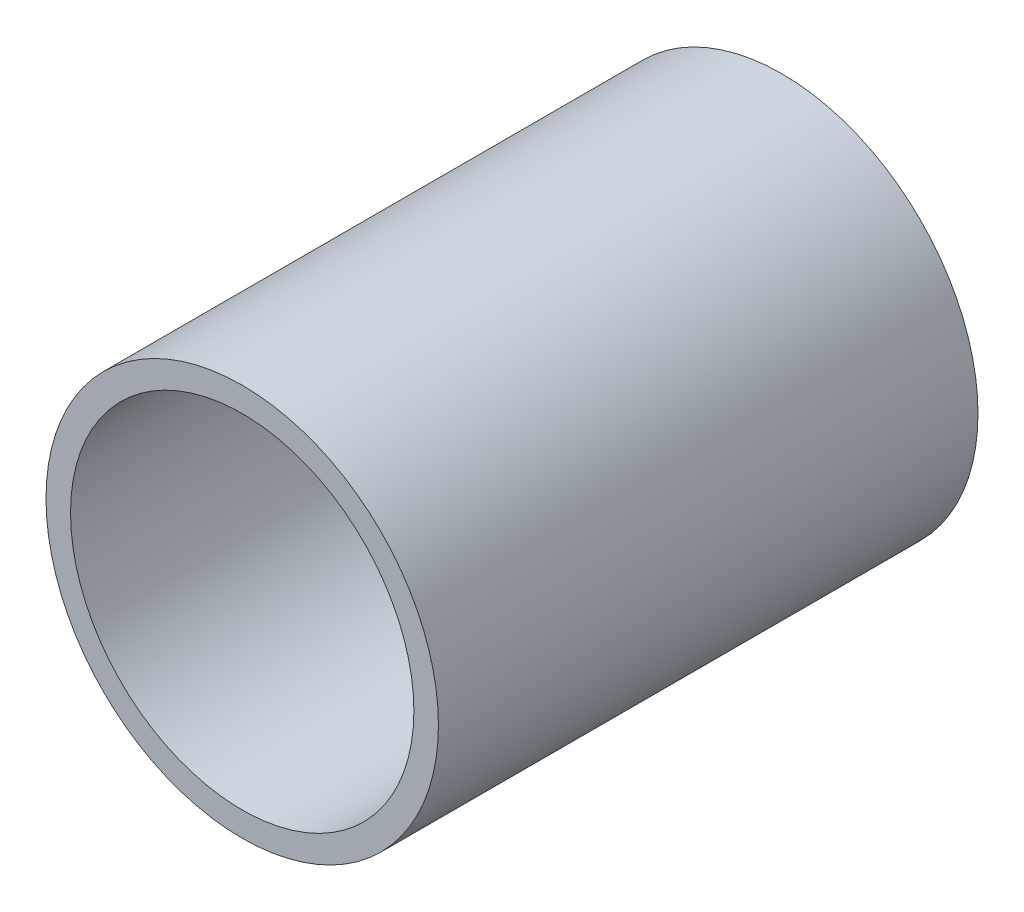
from build123d import *

# Parameters (mm, degrees)
SLEEVE_PROFILE_80X_70_R   = 40
SLEEVE_PROFILE_80X_70_R_2 = 35
SLEEVE_BODY_L110_DEPTH    = 110


with BuildPart() as part:
    # Sleeve Profile Ø80xØ70 → Sleeve Body L110 (new body)
    with BuildSketch(Plane.XY):
        Circle(SLEEVE_PROFILE_80X_70_R)
        Circle(SLEEVE_PROFILE_80X_70_R_2, mode=Mode.SUBTRACT)
    extrude(amount=SLEEVE_BODY_L110_DEPTH)


solid = part.part
